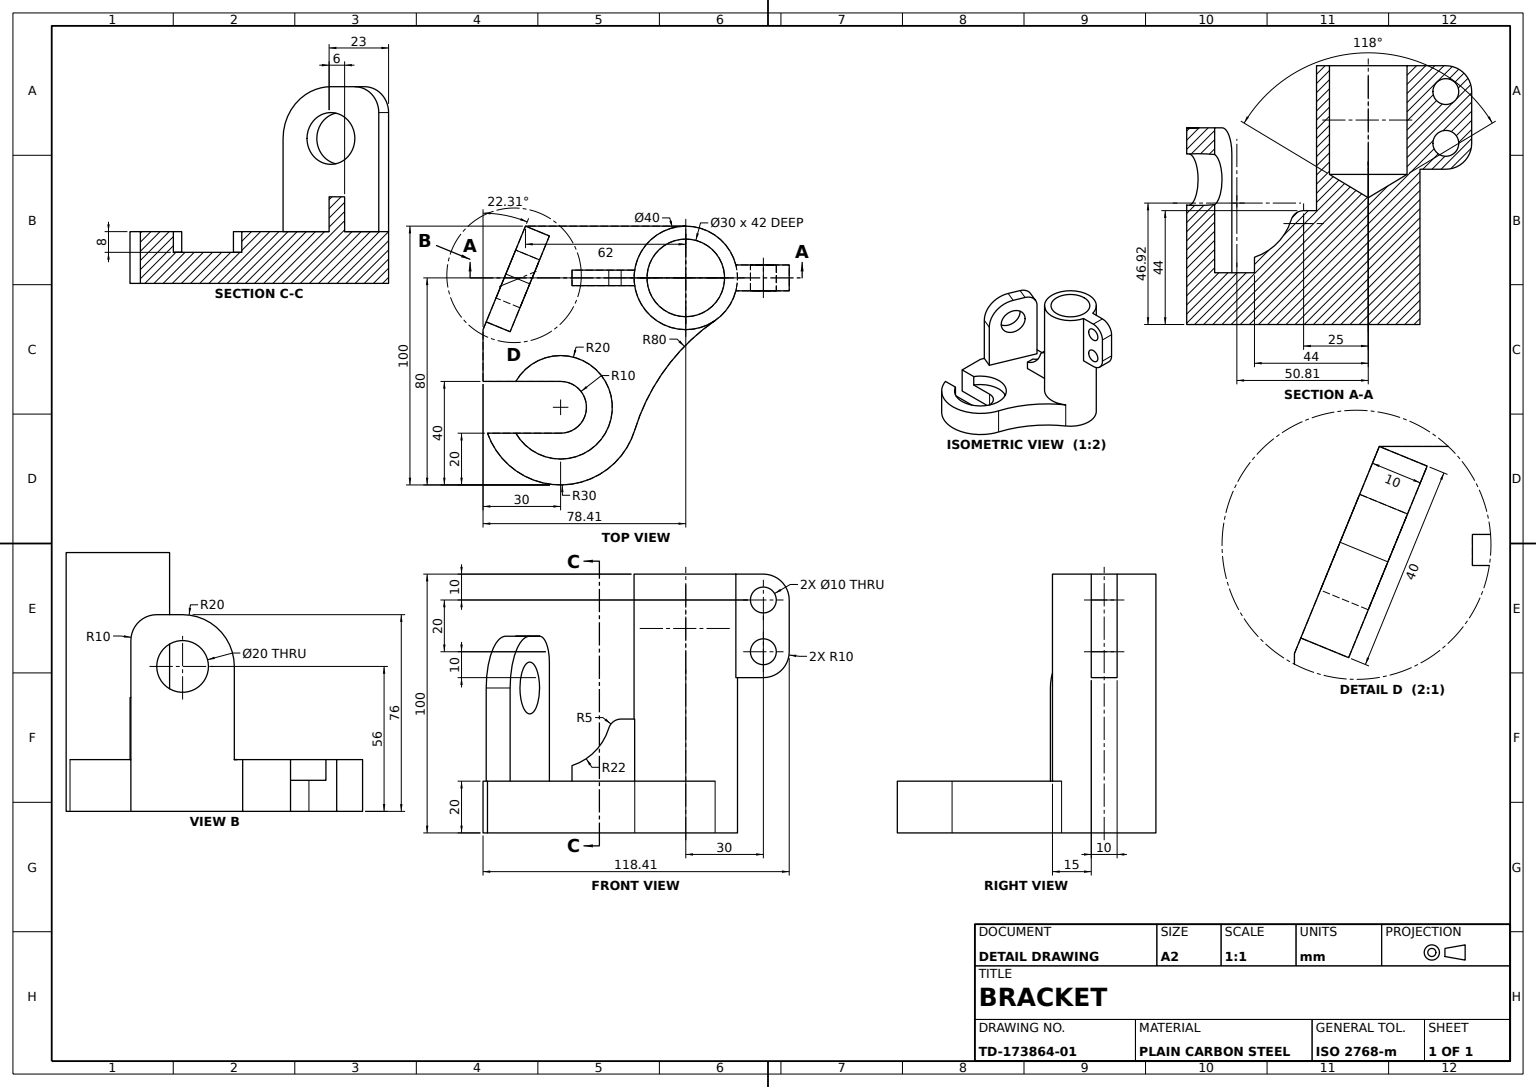
from build123d import *

# Parameters (mm, degrees)
COLUMN_PROFILE_SKETCH_R   = 20
COLUMN_BOSS_DEPTH         = 100
BASE_ARM_PLATE_DEPTH      = 20
COLUMN_BORE_30_D          = 30
COLUMN_BORE_30_DEPTH      = 42
COLUMN_BORE_30_TIP        = 9.012909285
HOOK_GUIDE_BLOCK_SKETCH_R = 10
HOOK_GUIDE_BLOCK_DEPTH    = 10
HOOK_SLOT_CUT_DEPTH       = 138.652199764
HOOK_RECESS_SKETCH_R      = 20
HOOK_RECESS_20_DEPTH      = 8
CLAMP_LUG_SKETCH_W        = 21.478013603
CLAMP_LUG_SKETCH_H        = 10
CLAMP_LUG_DEPTH           = 40
CLAMP_LUG_FILLET_R10_R    = 10
CLAMP_HOLES_SKETCH_R      = 5
CLAMP_HOLES_2X_10_DEPTH   = 40
EYE_LUG_DEPTH             = 3


with BuildPart() as part:
    # Column Profile Sketch → Column Boss (new body)
    with BuildSketch(Plane(origin=(0, 0, 0), x_dir=(1, 0, 0), z_dir=(0, 1, 0))):
        with Locations(Location((0, 0, 0), (0, 0, 270))):
            Circle(COLUMN_PROFILE_SKETCH_R)
    extrude(amount=COLUMN_BOSS_DEPTH)

    # Base Arm Profile Sketch → Base Arm Plate (add)
    with BuildSketch(Plane(origin=(0, 0, 0), x_dir=(1, 0, 0), z_dir=(0, 1, 0))):
        with BuildLine():
            Line((0, 20), (-62, 20))
            Line((-62, 20), (-78.41, -20))
            Line((-78.41, -20), (-78.41, -50))
            ThreePointArc((-78.41, -50), (-52.871711259, -79.666363657), (-19.737124491, -58.82418325))
            ThreePointArc((-19.737124491, -58.82418325), (-7.771853725, -35.023523327), (11.344775373, -16.471067717))
            ThreePointArc((11.344775373, -16.471067717), (-19.097399749, -5.9404817), (0, 20))
        make_face()
    extrude(amount=BASE_ARM_PLATE_DEPTH)

    # Column Bore Ø30
    with Locations(Plane.ZX.offset(100)):
        with Locations((0, 0)):
            Hole(COLUMN_BORE_30_D / 2, depth=COLUMN_BORE_30_DEPTH)
            with Locations((0, 0, -(COLUMN_BORE_30_DEPTH + COLUMN_BORE_30_TIP / 2))):  # 118° drill point
                Cone(0, COLUMN_BORE_30_D / 2, COLUMN_BORE_30_TIP, mode=Mode.SUBTRACT)

    # Hook Guide Block Sketch → Hook Guide Block (add)
    with BuildSketch(Plane(origin=(-60.091325676, 0, -24.652466359), x_dir=(-0.3795512800466907, 0, 0.9251707009060105), z_dir=(-0.9251707009060105, 0, -0.3795512800466907))):
        with BuildLine():
            Line((5.028765345, 20), (5.028765345, 66))
            ThreePointArc((5.028765345, 66), (7.957697533, 73.071067812), (15.028765345, 76))
            Line((15.028765345, 76), (25.028765345, 76))
            ThreePointArc((25.028765345, 76), (39.170900969, 70.142135624), (45.028765345, 56))
            Line((45.028765345, 56), (45.028765345, 20))
            Line((45.028765345, 20), (5.028765345, 20))
        make_face()
        with Locations((25.028765345, 56)):
            Circle(HOOK_GUIDE_BLOCK_SKETCH_R, mode=Mode.SUBTRACT)
    extrude(amount=-HOOK_GUIDE_BLOCK_DEPTH)

    # Hook Slot Sketch → Hook Slot Cut (cut, through all)
    with BuildSketch(Plane(origin=(0, 20, 0), x_dir=(1, 0, 0), z_dir=(0, 1, 0))):
        with BuildLine():
            Line((-48.41, -40), (-78.41, -40))
            Line((-78.41, -40), (-78.41, -60))
            Line((-78.41, -60), (-48.41, -60))
            ThreePointArc((-48.41, -60), (-38.41, -50), (-48.41, -40))
        make_face()
    extrude(amount=-HOOK_SLOT_CUT_DEPTH, mode=Mode.SUBTRACT)

    # Hook Recess Sketch → Hook Recess Ø20 (cut)
    with BuildSketch(Plane(origin=(0, 20, 0), x_dir=(1, 0, 0), z_dir=(0, 1, 0))):
        with Locations((-48.41, -50)):
            Circle(HOOK_RECESS_SKETCH_R)
    extrude(amount=-HOOK_RECESS_20_DEPTH, mode=Mode.SUBTRACT)

    # Clamp Lug Sketch → Clamp Lug (add)
    with BuildSketch(Plane(origin=(0, 100, 0), x_dir=(1, 0, 0), z_dir=(0, 1, 0))):
        with Locations((29.260993199, 0)):
            Rectangle(CLAMP_LUG_SKETCH_W, CLAMP_LUG_SKETCH_H)
    extrude(amount=-CLAMP_LUG_DEPTH)

    # Clamp Lug Fillet R10
    clamp_lug_fillet_r10_edges = [part.edges().sort_by_distance(p)[0] for p in [
        (40, 60, 0),
        (40, 100, 0),
    ]]
    fillet(clamp_lug_fillet_r10_edges, radius=CLAMP_LUG_FILLET_R10_R)

    # Clamp Holes Sketch → Clamp Holes 2xØ10 (cut)
    with BuildSketch(Plane.XY.offset(5)):
        with Locations((30, 90)):
            Circle(CLAMP_HOLES_SKETCH_R)
        with Locations((30, 70)):
            Circle(CLAMP_HOLES_SKETCH_R)
    extrude(amount=-CLAMP_HOLES_2X_10_DEPTH, mode=Mode.SUBTRACT)

    # Eye Lug Sketch → Eye Lug (add, symmetric)
    with BuildSketch(Plane.XY):
        with BuildLine():
            Line((-44, 20), (-44, 26))
            ThreePointArc((-44, 26), (-35.12324798, 31.496493808), (-29.780131863, 40.466403549))
            ThreePointArc((-29.780131863, 40.466403549), (-27.972203076, 43.020697561), (-25, 44))
            Line((-25, 44), (-20, 44))
            Line((-20, 44), (-17, 44))
            Line((-17, 44), (-17, 20))
            Line((-17, 20), (-44, 20))
        make_face()
    extrude(amount=EYE_LUG_DEPTH, both=True)


solid = part.part
